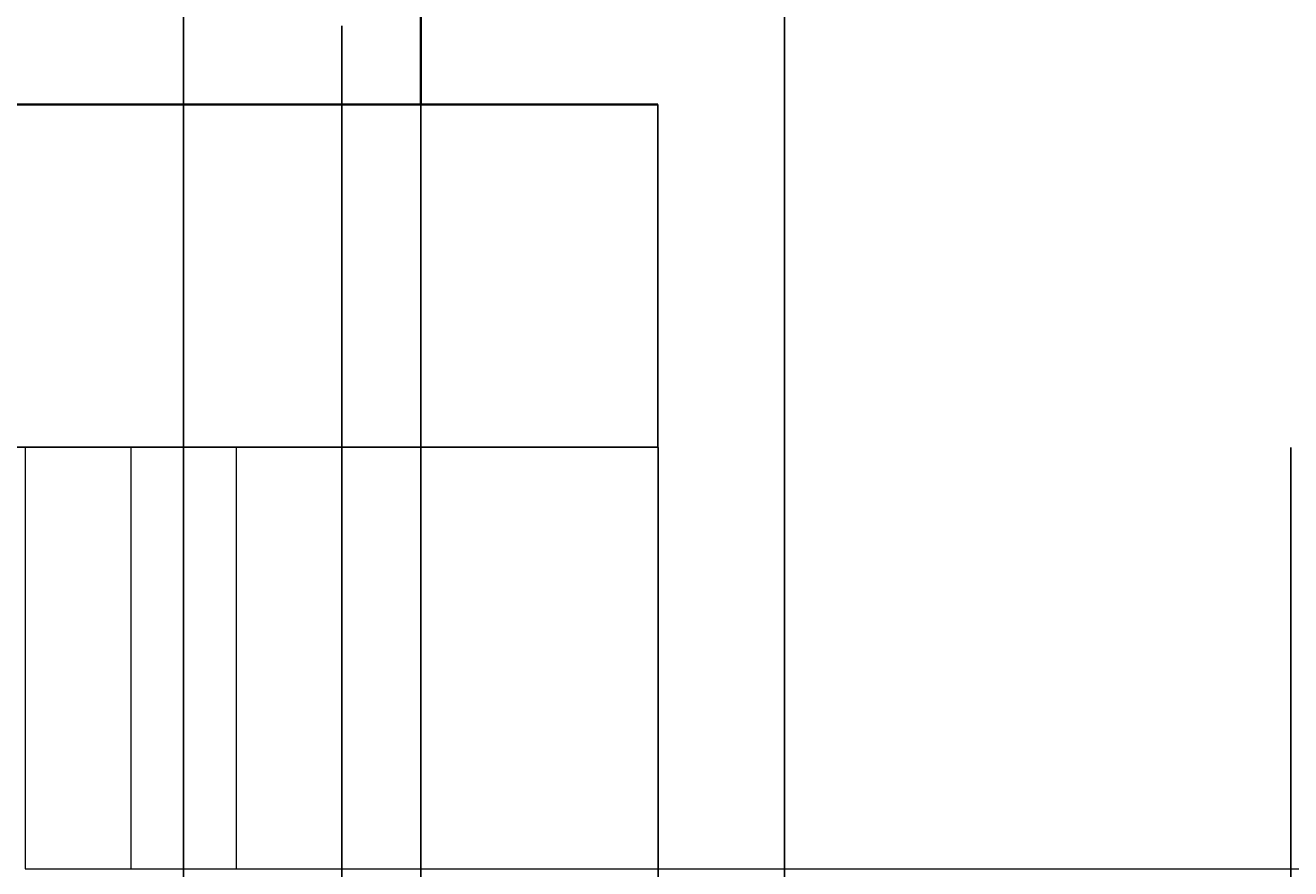
# Model space of a CAD drawing. Units: inches. Extents: x 867 to 1667, y -234 to 788.
# Tile 16 of 42: x 1212 to 1356, y -104 to -8. Entities that reach past the tile are written whole.
import ezdxf

# ---------------------------------------------------------------- set-up
doc = ezdxf.new("R2010")
doc.units = ezdxf.units.IN
doc.header["$MEASUREMENT"] = 0
for name, color, linetype, lineweight in [('A-ANNO-DIMS', 2, 'Continuous', 18), ('A-FLOR-OTLN', 7, 'Continuous', 25), ('A-FLOR-STRS', 7, 'Continuous', 18), ('A-Wall', 7, 'Continuous', 35)]:
    doc.layers.add(name, color=color, linetype=linetype, lineweight=lineweight)
doc.styles.get("Standard").update_dxf_attribs({"font": 'arial.ttf'})
doc.dimstyles.get("Standard").update_dxf_attribs({"dimtxt": 0.6875, "dimasz": 0.18, "dimexe": 0.18, "dimexo": 0.0625, "dimgap": 0.09, "dimtad": 0, "dimdec": 4, "dimzin": 0, "dimdsep": 46, "dimlunit": 4, "dimtxsty": 'Standard', "dimcen": 0.09, "dimadec": 0, "dimazin": 0, "dimtfac": 1, "dimtdec": 4, "dimtofl": 0, "dimtmove": 0, "dimatfit": 3, "dimfxl": 1, "dimtolj": 1, "dimtzin": 0, "dimarcsym": 0})

# ---------------------------------------------------------------- blocks, each defined once
blk = doc.blocks.new('*D27')
at = {"layer": 'A-ANNO-DIMS', "color": 0, "lineweight": -2, "transparency": 16777216}
for p, q in [((1070.89, -55.97), (1070.89, -233.54)), ((1525.26, -186.47), (1525.26, -233.54)), ((1071.07, -233.36), (1296.81, -233.36)), ((1525.08, -233.36), (1299.34, -233.36))]:
    blk.add_line(p, q, dxfattribs=at)
at = {"layer": 'A-ANNO-DIMS', "color": 0, "transparency": 16777216}
for points in [[(1071.07, -233.33), (1071.07, -233.39), (1070.89, -233.36)], [(1525.08, -233.33), (1525.08, -233.39), (1525.26, -233.36)]]:
    blk.add_solid(points, dxfattribs=at)
at = {"layer": 'Defpoints', "color": 0, "transparency": 16777216}
for p in [(1070.89, -55.91), (1525.26, -186.41), (1525.26, -233.36)]:
    blk.add_point(p, dxfattribs=at)
at = {"layer": 'A-ANNO-DIMS', "color": 0, "transparency": 16777216, "insert": (1298.08, -233.36), "char_height": 0.688, "attachment_point": 5}
blk.add_mtext('\\A1;454.4', dxfattribs=at)
blk = doc.blocks.new('*D30')
at = {"layer": 'A-ANNO-DIMS', "color": 0, "lineweight": -2, "transparency": 16777216}
for p, q in [((1229.89, 623.55), (1229.89, -233.54)), ((1298.3, 623.55), (1298.3, -233.54)), ((1230.07, -233.36), (1262.91, -233.36)), ((1298.12, -233.36), (1265.28, -233.36))]:
    blk.add_line(p, q, dxfattribs=at)
at = {"layer": 'A-ANNO-DIMS', "color": 0, "transparency": 16777216}
for points in [[(1230.07, -233.33), (1230.07, -233.39), (1229.89, -233.36)], [(1298.12, -233.33), (1298.12, -233.39), (1298.3, -233.36)]]:
    blk.add_solid(points, dxfattribs=at)
at = {"layer": 'Defpoints', "color": 0, "transparency": 16777216}
for p in [(1229.89, 623.62), (1298.3, 623.62), (1298.3, -233.36)]:
    blk.add_point(p, dxfattribs=at)
at = {"layer": 'A-ANNO-DIMS', "color": 0, "transparency": 16777216, "insert": (1264.09, -233.36), "char_height": 0.688, "attachment_point": 5}
blk.add_mtext('\\A1;68.41', dxfattribs=at)
blk = doc.blocks.new('*D45')
at = {"layer": 'A-ANNO-DIMS', "color": 0, "lineweight": -2, "transparency": 16777216}
for p, q in [((1079.89, -7.95), (1079.89, -233.54)), ((1247.89, -7.95), (1247.89, -233.54)), ((1080.07, -233.36), (1163.07, -233.36)), ((1247.71, -233.36), (1164.7, -233.36))]:
    blk.add_line(p, q, dxfattribs=at)
at = {"layer": 'A-ANNO-DIMS', "color": 0, "transparency": 16777216}
for points in [[(1080.07, -233.33), (1080.07, -233.39), (1079.89, -233.36)], [(1247.71, -233.33), (1247.71, -233.39), (1247.89, -233.36)]]:
    blk.add_solid(points, dxfattribs=at)
at = {"layer": 'Defpoints', "color": 0, "transparency": 16777216}
for p in [(1079.89, -7.88), (1247.89, -7.88), (1247.89, -233.36)]:
    blk.add_point(p, dxfattribs=at)
at = {"layer": 'A-ANNO-DIMS', "color": 0, "transparency": 16777216, "insert": (1163.89, -233.36), "char_height": 0.688, "attachment_point": 5}
blk.add_mtext('\\A1;168', dxfattribs=at)
blk = doc.blocks.new('*D46')
at = {"layer": 'A-ANNO-DIMS', "color": 0, "lineweight": -2, "transparency": 16777216}
for p, q in [((1256.89, -16.95), (1256.89, -233.54)), ((1394.89, -16.95), (1394.89, -233.54)), ((1257.07, -233.36), (1325.07, -233.36)), ((1394.71, -233.36), (1326.7, -233.36))]:
    blk.add_line(p, q, dxfattribs=at)
at = {"layer": 'A-ANNO-DIMS', "color": 0, "transparency": 16777216}
for points in [[(1257.07, -233.33), (1257.07, -233.39), (1256.89, -233.36)], [(1394.71, -233.33), (1394.71, -233.39), (1394.89, -233.36)]]:
    blk.add_solid(points, dxfattribs=at)
at = {"layer": 'Defpoints', "color": 0, "transparency": 16777216}
for p in [(1256.89, -16.88), (1394.89, -16.88), (1394.89, -233.36)]:
    blk.add_point(p, dxfattribs=at)
at = {"layer": 'A-ANNO-DIMS', "color": 0, "transparency": 16777216, "insert": (1325.89, -233.36), "char_height": 0.688, "attachment_point": 5}
blk.add_mtext('\\A1;138', dxfattribs=at)
blk = doc.blocks.new('*D48')
at = {"layer": 'A-ANNO-DIMS', "color": 0, "lineweight": -2, "transparency": 16777216}
for p, q in [((1283.89, -55.97), (1283.89, -233.54)), ((1355.89, -55.97), (1355.89, -233.54)), ((1284.07, -233.36), (1319.31, -233.36)), ((1355.71, -233.36), (1320.46, -233.36))]:
    blk.add_line(p, q, dxfattribs=at)
at = {"layer": 'A-ANNO-DIMS', "color": 0, "transparency": 16777216}
for points in [[(1284.07, -233.33), (1284.07, -233.39), (1283.89, -233.36)], [(1355.71, -233.33), (1355.71, -233.39), (1355.89, -233.36)]]:
    blk.add_solid(points, dxfattribs=at)
at = {"layer": 'Defpoints', "color": 0, "transparency": 16777216}
for p in [(1283.89, -55.91), (1355.89, -55.91), (1355.89, -233.36)]:
    blk.add_point(p, dxfattribs=at)
at = {"layer": 'A-ANNO-DIMS', "color": 0, "transparency": 16777216, "insert": (1319.89, -233.36), "char_height": 0.688, "attachment_point": 5}
blk.add_mtext('\\A1;72', dxfattribs=at)
blk = doc.blocks.new('*D62')
at = {"layer": 'A-ANNO-DIMS', "color": 0, "lineweight": -2, "transparency": 16777216}
for p, q in [((1247.89, -55.97), (1247.89, -233.54)), ((1283.89, -55.97), (1283.89, -233.54)), ((1248.07, -233.36), (1265.3, -233.36)), ((1283.71, -233.36), (1266.47, -233.36))]:
    blk.add_line(p, q, dxfattribs=at)
at = {"layer": 'A-ANNO-DIMS', "color": 0, "transparency": 16777216}
for points in [[(1248.07, -233.33), (1248.07, -233.39), (1247.89, -233.36)], [(1283.71, -233.33), (1283.71, -233.39), (1283.89, -233.36)]]:
    blk.add_solid(points, dxfattribs=at)
at = {"layer": 'Defpoints', "color": 0, "transparency": 16777216}
for p in [(1247.89, -55.91), (1283.89, -55.91), (1247.89, -233.36)]:
    blk.add_point(p, dxfattribs=at)
at = {"layer": 'A-ANNO-DIMS', "color": 0, "transparency": 16777216, "insert": (1265.89, -233.36), "char_height": 0.688, "attachment_point": 5}
blk.add_mtext('\\A1;36', dxfattribs=at)

msp = doc.modelspace()

# ---------------------------------------------------------------- linework, layer by layer
at = {"layer": 'A-FLOR-OTLN'}
for p in [(1283.8866, -16.883), (1070.8866, -55.9081)]:
    msp.add_line(p, (1283.8866, -55.9081), dxfattribs=at)
at = {"layer": 'A-FLOR-STRS'}
for p, q in [((1211.8866, -55.9081), (1211.8866, -103.9081)), ((1223.8866, -55.9081), (1223.8866, -103.9081)), ((1235.8866, -55.9081), (1235.8866, -103.9081)), ((1247.8866, -55.9081), (1247.8866, -103.9081)), ((1211.8866, -103.9081), (1427.8866, -103.9081))]:
    msp.add_line(p, q, dxfattribs=at)
at = {"layer": 'A-Wall'}
for p, q in [((1256.8866, 101.9059), (1256.8866, -16.883)), ((1283.8866, -16.883), (1070.8866, -16.883))]:
    msp.add_line(p, q, dxfattribs=at)

# ---------------------------------------------------------------- dimensions: what is measured, and where the dimension line sits
at = {"layer": 'A-ANNO-DIMS'}
for base, p1, p2, override, picture, middle in [((1298.2966, -233.3581), (1229.8866, 623.617), (1298.2966, 623.617), {"dimdec": 2, "dimlfac": 1, "dimrnd": 0, "dimzin": 0, "dimdsep": 46, "dimlunit": 2}, '*D30', (1264.0916, -233.3581)), ((1247.8866, -233.3581), (1079.8866, -7.883), (1247.8866, -7.883), {"dimdec": 0, "dimlfac": 1, "dimrnd": 0, "dimzin": 0, "dimdsep": 46, "dimlunit": 2}, '*D45', (1163.8866, -233.3581)), ((1394.8866, -233.3581), (1256.8866, -16.883), (1394.8866, -16.883), {"dimdec": 0, "dimlfac": 1, "dimrnd": 0, "dimzin": 0, "dimdsep": 46, "dimlunit": 2}, '*D46', (1325.8866, -233.3581)), ((1525.2648, -233.3581), (1070.8866, -55.9081), (1525.2648, -186.4081), {"dimdec": 1, "dimlfac": 1, "dimrnd": 0, "dimzin": 0, "dimdsep": 46, "dimlunit": 2}, '*D27', (1298.0757, -233.3581)), ((1247.8866, -233.3581), (1283.8866, -55.9081), (1247.8866, -55.9081), {"dimdec": 0, "dimlfac": 1, "dimrnd": 0, "dimzin": 0, "dimdsep": 46, "dimlunit": 2}, '*D62', (1265.8866, -233.3581)), ((1355.8866, -233.3581), (1283.8866, -55.9081), (1355.8866, -55.9081), {"dimdec": 0, "dimlfac": 1, "dimrnd": 0, "dimzin": 0, "dimdsep": 46, "dimlunit": 2}, '*D48', (1319.8866, -233.3581))]:
    dim = msp.add_linear_dim(base=base, p1=p1, p2=p2, dimstyle='Standard', override=override, dxfattribs=at)
    dim.commit()
    dim.dimension.update_dxf_attribs({"geometry": picture, "text_midpoint": middle})

doc.saveas('drawing.dxf')
